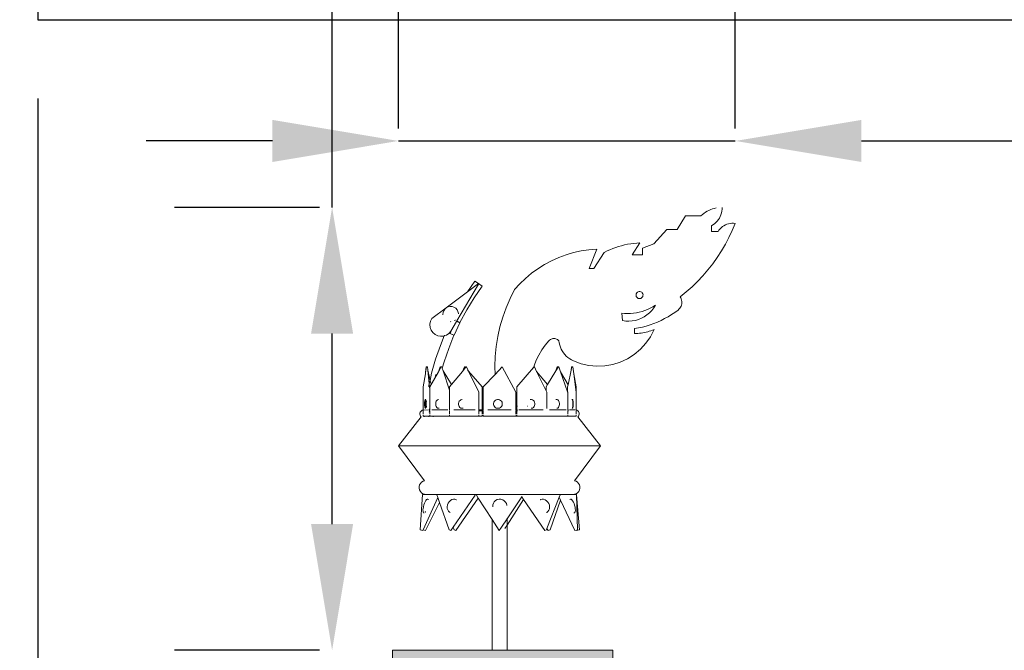
# Model space of a CAD drawing. Units: millimetres. Extents: x 7894 to 8038, y 6851 to 6951.
# Tile 44 of 49: x 7942.814 to 7950.619, y 6931.885 to 6936.88. Entities that reach past the tile are written whole.
import ezdxf

# ---------------------------------------------------------------- set-up
doc = ezdxf.new("R2010")
doc.units = ezdxf.units.MM
for name, color, linetype, lineweight in [('A-ANNO-DIMS', 2, 'Continuous', 18), ('A-FURN-ACCS', 8, 'Continuous', 13), ('A-FURN-SHLF', 7, 'Continuous', 30)]:
    doc.layers.add(name, color=color, linetype=linetype, lineweight=lineweight)
doc.layers.add('A-FURN-ACCS-PATT', color=116, linetype='Continuous', lineweight=9, true_color=0x136734)
doc.styles.get("Standard").update_dxf_attribs({"font": 'arial.ttf'})
doc.dimstyles.new('ISO-25', dxfattribs={"dimtxt": 1, "dimasz": 1, "dimexe": 1.25, "dimexo": 0.625, "dimtad": 1, "dimdec": 0, "dimlunit": 4, "dimtxsty": 'Standard', "dimcen": 2.5, "dimclrt": 1, "dimadec": 0, "dimazin": 0, "dimtfac": 1, "dimtdec": 0, "dimtmove": 0, "dimatfit": 3, "dimfxl": 1, "dimarcsym": 0})

# ---------------------------------------------------------------- blocks, each defined once
blk = doc.blocks.new('FLOATING-SHELF-ELEV')
for p, q in [((0, 0.5), (0, 0)), ((0, 0), (17.3035, 0))]:
    blk.add_line(p, q)
blk = doc.blocks.new('DISPLAY-LEAF-FINIAL')
for p, q in [((2.2094, 3.3343), (2.2756, 3.4413)), ((2.2756, 3.4413), (2.398, 3.4413)), ((2.398, 3.4413), (2.4094, 3.4516)), ((2.4094, 3.4516), (2.4214, 3.4612)), ((2.4214, 3.4612), (2.4341, 3.4699)), ((2.4341, 3.4699), (2.4472, 3.4778)), ((2.4472, 3.4778), (2.4609, 3.4849)), ((2.4609, 3.4849), (2.475, 3.4911)), ((2.475, 3.4911), (2.4894, 3.4964)), ((2.4894, 3.4964), (2.5041, 3.5007)), ((2.5041, 3.5007), (2.5191, 3.5041)), ((2.5507, 3.4368), (2.5438, 3.4237)), ((2.5562, 3.4504), (2.5507, 3.4368)), ((2.5605, 3.4646), (2.5562, 3.4504)), ((2.5634, 3.479), (2.5605, 3.4646)), ((2.5649, 3.4937), (2.5634, 3.479)), ((2.565, 3.5085), (2.5649, 3.4937)), ((2.4932, 3.3709), (2.4804, 3.3635)), ((2.4804, 3.3635), (2.4804, 3.3164)), ((2.5053, 3.3794), (2.4932, 3.3709)), ((2.5164, 3.3891), (2.5053, 3.3794)), ((2.5266, 3.3997), (2.5164, 3.3891)), ((2.5358, 3.4113), (2.5266, 3.3997)), ((2.5438, 3.4237), (2.5358, 3.4113)), ((2.5687, 3.3558), (2.5799, 3.3633)), ((2.5799, 3.3633), (2.5917, 3.3696)), ((2.5917, 3.3696), (2.604, 3.3748)), ((2.604, 3.3748), (2.6168, 3.3788)), ((2.6168, 3.3788), (2.63, 3.3815)), ((2.63, 3.3815), (2.6433, 3.3829)), ((2.6433, 3.3829), (2.6567, 3.3831)), ((2.6701, 3.3819), (2.6462, 3.3254)), ((2.6567, 3.3831), (2.6701, 3.3819)), ((2.0233, 3.2209), (2.1272, 3.3343)), ((2.1272, 3.3343), (2.2094, 3.3343)), ((2.4804, 3.3164), (2.5329, 3.3164)), ((2.5329, 3.3164), (2.5404, 3.3275)), ((2.5404, 3.3275), (2.5489, 3.3378)), ((2.5489, 3.3378), (2.5584, 3.3473)), ((2.5584, 3.3473), (2.5687, 3.3558)), ((2.6462, 3.3254), (2.6199, 3.27)), ((1.7453, 3.1982), (1.7688, 3.2049)), ((1.7688, 3.2049), (1.7926, 3.2108)), ((1.7926, 3.2108), (1.8166, 3.2158)), ((1.8166, 3.2158), (1.8408, 3.2199)), ((1.8408, 3.2199), (1.8651, 3.2232)), ((1.9139, 3.2271), (1.8536, 3.1329)), ((1.8651, 3.2232), (1.8895, 3.2256)), ((1.8895, 3.2256), (1.9139, 3.2271)), ((1.934, 3.1854), (2.0233, 3.2209)), ((2.5912, 3.2159), (2.56, 3.1631)), ((2.6199, 3.27), (2.5912, 3.2159)), ((1.2698, 3.1109), (1.3282, 3.1326)), ((1.3282, 3.1326), (1.3879, 3.1503)), ((1.3879, 3.1503), (1.4487, 3.1639)), ((1.4487, 3.1639), (1.5102, 3.1734)), ((1.5102, 3.1734), (1.5723, 3.1786)), ((1.5723, 3.1786), (1.5113, 3.0242)), ((1.5498, 3.0242), (1.6318, 3.1522)), ((1.6318, 3.1522), (1.6538, 3.163)), ((1.6538, 3.163), (1.6762, 3.173)), ((1.6762, 3.173), (1.6989, 3.1822)), ((1.6989, 3.1822), (1.7219, 3.1906)), ((1.7219, 3.1906), (1.7453, 3.1982)), ((1.8536, 3.1329), (1.934, 3.1329)), ((1.934, 3.1329), (1.934, 3.1854)), ((2.56, 3.1631), (2.5265, 3.1117)), ((1.1053, 3.0227), (1.1581, 3.0558)), ((1.1581, 3.0558), (1.213, 3.0852)), ((1.213, 3.0852), (1.2698, 3.1109)), ((2.4908, 3.0619), (2.4529, 3.0137)), ((2.5265, 3.1117), (2.4908, 3.0619)), ((1.0071, 2.9462), (1.0549, 2.9861)), ((1.0549, 2.9861), (1.1053, 3.0227)), ((1.5113, 3.0242), (1.5498, 3.0242)), ((2.4129, 2.9672), (2.3708, 2.9226)), ((2.4529, 3.0137), (2.4129, 2.9672)), ((0.634, 2.9001), (0.4633, 2.6089)), ((0.6052, 2.9243), (0.5471, 2.8395)), ((0.634, 2.9046), (0.5471, 2.8395)), ((0.634, 2.9046), (0.6052, 2.9243)), ((0.634, 2.9001), (0.634, 2.9046)), ((0.6629, 2.8848), (0.634, 2.9046)), ((0.9202, 2.857), (0.9622, 2.9031)), ((0.9622, 2.9031), (1.0071, 2.9462)), ((2.3708, 2.9226), (2.3268, 2.8799)), ((0.5471, 2.8395), (0.379, 2.7129)), ((0.5989, 2.7915), (0.6629, 2.8848)), ((0.9202, 2.857), (0.8844, 2.7861)), ((1.8829, 2.8172), (1.8849, 2.8243)), ((1.8829, 2.8099), (1.8829, 2.8172)), ((1.8849, 2.8243), (1.8885, 2.8306)), ((1.8885, 2.8306), (1.8937, 2.8357)), ((1.8937, 2.8357), (1.9001, 2.8393)), ((1.9001, 2.8393), (1.9071, 2.8412)), ((1.9071, 2.8412), (1.9144, 2.8411)), ((1.9144, 2.8411), (1.9215, 2.8392)), ((1.9215, 2.8392), (1.9278, 2.8355)), ((1.9278, 2.8355), (1.9329, 2.8303)), ((1.9329, 2.8303), (1.9365, 2.824)), ((1.9365, 2.824), (1.9384, 2.8169)), ((1.9384, 2.8169), (1.9383, 2.8096)), ((2.281, 2.8392), (2.2333, 2.8006)), ((2.3268, 2.8799), (2.281, 2.8392)), ((0.5406, 2.6956), (0.5989, 2.7915)), ((0.8844, 2.7861), (0.853, 2.7132)), ((1.8847, 2.8029), (1.8829, 2.8099)), ((1.8884, 2.7965), (1.8847, 2.8029)), ((1.8935, 2.7913), (1.8884, 2.7965)), ((1.8998, 2.7877), (1.8935, 2.7913)), ((1.9068, 2.7857), (1.8998, 2.7877)), ((1.9141, 2.7857), (1.9068, 2.7857)), ((1.9212, 2.7875), (1.9141, 2.7857)), ((1.9275, 2.7912), (1.9212, 2.7875)), ((1.9327, 2.7963), (1.9275, 2.7912)), ((1.9364, 2.8026), (1.9327, 2.7963)), ((1.9383, 2.8096), (1.9364, 2.8026)), ((2.0364, 2.7343), (2.0167, 2.7218)), ((2.0364, 2.7343), (2.023, 2.7124)), ((2.2333, 2.8006), (2.2382, 2.7921)), ((2.2382, 2.7921), (2.242, 2.7831)), ((2.243, 2.7351), (2.2397, 2.7259)), ((2.242, 2.7831), (2.2446, 2.7737)), ((2.2452, 2.7446), (2.243, 2.7351)), ((2.2446, 2.7737), (2.246, 2.764)), ((2.2462, 2.7543), (2.2452, 2.7446)), ((2.246, 2.764), (2.2462, 2.7543)), ((0.379, 2.7129), (0.2638, 2.6275)), ((0.3526, 2.6596), (0.3535, 2.675)), ((0.3527, 2.6591), (0.3526, 2.6596)), ((0.3526, 2.6569), (0.3527, 2.6591)), ((0.3535, 2.675), (0.3584, 2.6897)), ((0.3584, 2.6897), (0.3671, 2.7026)), ((0.3671, 2.7026), (0.379, 2.7129)), ((0.379, 2.7129), (0.3932, 2.7199)), ((0.3932, 2.7199), (0.4088, 2.7231)), ((0.4088, 2.7231), (0.4248, 2.7223)), ((0.4248, 2.7223), (0.44, 2.7176)), ((0.44, 2.7176), (0.4533, 2.7092)), ((0.4533, 2.7092), (0.464, 2.6977)), ((0.464, 2.6977), (0.4713, 2.6839)), ((0.4713, 2.6839), (0.4746, 2.6689)), ((0.4745, 2.6667), (0.4746, 2.6689)), ((0.4745, 2.6667), (0.4746, 2.6661)), ((0.5406, 2.6956), (0.4875, 2.5967)), ((0.853, 2.7132), (0.8261, 2.6384)), ((1.793, 2.6675), (1.7698, 2.6695)), ((1.7698, 2.6695), (1.7755, 2.6114)), ((1.8164, 2.6669), (1.793, 2.6675)), ((1.8397, 2.6677), (1.8164, 2.6669)), ((1.863, 2.6698), (1.8397, 2.6677)), ((1.886, 2.6733), (1.863, 2.6698)), ((1.9089, 2.6781), (1.886, 2.6733)), ((1.9314, 2.6843), (1.9089, 2.6781)), ((1.9535, 2.6918), (1.9314, 2.6843)), ((1.97, 2.6568), (1.9487, 2.6423)), ((1.9751, 2.7005), (1.9535, 2.6918)), ((1.9896, 2.6734), (1.97, 2.6568)), ((1.9962, 2.7106), (1.9751, 2.7005)), ((2.0073, 2.692), (1.9896, 2.6734)), ((2.0167, 2.7218), (1.9962, 2.7106)), ((2.023, 2.7124), (2.0073, 2.692)), ((2.1643, 2.6592), (2.1374, 2.6427)), ((2.1904, 2.6768), (2.1643, 2.6592)), ((2.2158, 2.6954), (2.1904, 2.6768)), ((2.2231, 2.7019), (2.2158, 2.6954)), ((2.2296, 2.7092), (2.2231, 2.7019)), ((2.2352, 2.7172), (2.2296, 2.7092)), ((2.2397, 2.7259), (2.2352, 2.7172)), ((0.2535, 2.6069), (0.2491, 2.5845)), ((0.2491, 2.58), (0.2491, 2.5845)), ((0.2491, 2.58), (0.2508, 2.5572)), ((0.2638, 2.6275), (0.2535, 2.6069)), ((0.4145, 2.6055), (0.4132, 2.6029)), ((0.4608, 2.6047), (0.4152, 2.527)), ((0.4402, 2.4957), (0.4858, 2.593)), ((0.4431, 2.613), (0.4459, 2.6117)), ((0.4509, 2.6151), (0.4489, 2.6161)), ((0.4633, 2.6089), (0.4608, 2.6047)), ((0.4858, 2.593), (0.4608, 2.6047)), ((0.4633, 2.6089), (0.4875, 2.5967)), ((0.8261, 2.6384), (0.804, 2.5621)), ((1.801, 2.6079), (1.7755, 2.6114)), ((1.8266, 2.607), (1.801, 2.6079)), ((1.8523, 2.6088), (1.8266, 2.607)), ((1.8776, 2.6133), (1.8523, 2.6088)), ((1.9023, 2.6204), (1.8776, 2.6133)), ((1.9261, 2.6301), (1.9023, 2.6204)), ((1.9487, 2.6423), (1.9261, 2.6301)), ((1.9942, 2.5779), (1.9641, 2.5686)), ((2.0239, 2.5884), (1.9942, 2.5779)), ((2.0531, 2.6002), (2.0239, 2.5884)), ((2.0818, 2.6131), (2.0531, 2.6002)), ((2.1099, 2.6273), (2.0818, 2.6131)), ((2.1374, 2.6427), (2.1099, 2.6273)), ((0.2508, 2.5572), (0.2586, 2.5356)), ((0.2586, 2.5356), (0.2719, 2.5167)), ((0.2719, 2.5167), (0.2898, 2.5018)), ((0.2898, 2.5018), (0.3111, 2.4919)), ((0.3802, 2.4968), (0.3998, 2.5097)), ((0.3983, 2.5132), (0.4016, 2.5117)), ((0.3998, 2.5097), (0.4016, 2.5117)), ((0.4029, 2.5132), (0.4004, 2.5144)), ((0.4016, 2.5117), (0.4029, 2.5132)), ((0.4016, 2.5117), (0.4399, 2.495)), ((0.4029, 2.5132), (0.4152, 2.527)), ((0.4029, 2.5132), (0.4402, 2.4957)), ((0.4085, 2.5106), (0.4078, 2.509)), ((0.4202, 2.5355), (0.4085, 2.5106)), ((0.804, 2.5621), (0.7866, 2.4847)), ((1.9029, 2.5538), (1.8718, 2.5484)), ((1.8718, 2.5484), (1.8718, 2.5082)), ((1.8718, 2.5082), (1.885, 2.5088)), ((1.885, 2.5088), (1.8981, 2.5098)), ((1.8981, 2.5098), (1.9112, 2.5112)), ((1.9336, 2.5606), (1.9029, 2.5538)), ((1.9112, 2.5112), (1.9243, 2.513)), ((1.9243, 2.513), (1.9373, 2.5152)), ((1.9641, 2.5686), (1.9336, 2.5606)), ((1.9373, 2.5152), (1.9502, 2.5177)), ((1.9502, 2.5177), (1.9631, 2.5206)), ((1.9631, 2.5206), (1.9758, 2.5239)), ((1.9758, 2.5239), (1.9885, 2.5276)), ((1.9885, 2.5276), (2.001, 2.5317)), ((2.0257, 2.5409), (1.9968, 2.4843)), ((2.001, 2.5317), (2.0134, 2.5361)), ((2.0134, 2.5361), (2.0257, 2.5409)), ((0.3111, 2.4919), (0.3343, 2.4876)), ((0.3628, 2.4909), (0.3323, 2.4155)), ((0.3343, 2.4876), (0.3579, 2.4893)), ((0.3579, 2.4893), (0.3628, 2.4909)), ((0.3628, 2.4909), (0.3802, 2.4968)), ((0.3649, 2.4962), (0.3628, 2.4909)), ((0.3978, 2.391), (0.4399, 2.495)), ((0.7866, 2.4847), (0.774, 2.4062)), ((1.1928, 2.4521), (1.1631, 2.4165)), ((1.1981, 2.4572), (1.1928, 2.4521)), ((1.2041, 2.4615), (1.1981, 2.4572)), ((1.2106, 2.465), (1.2041, 2.4615)), ((1.2175, 2.4675), (1.2106, 2.465)), ((1.2247, 2.469), (1.2175, 2.4675)), ((1.2321, 2.4695), (1.2247, 2.469)), ((1.2395, 2.469), (1.2321, 2.4695)), ((1.2467, 2.4675), (1.2395, 2.469)), ((1.2536, 2.465), (1.2467, 2.4675)), ((1.2601, 2.4615), (1.2536, 2.465)), ((1.2661, 2.4572), (1.2601, 2.4615)), ((1.2714, 2.4521), (1.2661, 2.4572)), ((1.274, 2.435), (1.2714, 2.4521)), ((1.278, 2.4183), (1.274, 2.435)), ((1.9607, 2.4321), (1.918, 2.3851)), ((1.9968, 2.4843), (1.9607, 2.4321)), ((0.3323, 2.4155), (0.2946, 2.3057)), ((0.3614, 2.2848), (0.3978, 2.391)), ((0.774, 2.4062), (0.7662, 2.3272)), ((1.1364, 2.3787), (1.1127, 2.339)), ((1.1631, 2.4165), (1.1364, 2.3787)), ((1.2834, 2.4019), (1.278, 2.4183)), ((1.2903, 2.3861), (1.2834, 2.4019)), ((1.2985, 2.371), (1.2903, 2.3861)), ((1.308, 2.3566), (1.2985, 2.371)), ((1.3187, 2.3431), (1.308, 2.3566)), ((1.3305, 2.3306), (1.3187, 2.3431)), ((1.8695, 2.3441), (1.8161, 2.3099)), ((1.918, 2.3851), (1.8695, 2.3441)), ((0.2946, 2.3057), (0.263, 2.1941)), ((0.3472, 2.2349), (0.3614, 2.2848)), ((0.7662, 2.3272), (0.7634, 2.2478)), ((1.0923, 2.2975), (1.0752, 2.2545)), ((1.1127, 2.339), (1.0923, 2.2975)), ((1.3434, 2.3192), (1.3305, 2.3306)), ((1.3572, 2.3089), (1.3434, 2.3192)), ((1.3719, 2.2999), (1.3572, 2.3089)), ((1.3873, 2.2921), (1.3719, 2.2999)), ((1.4469, 2.2701), (1.3873, 2.2921)), ((1.5088, 2.256), (1.4469, 2.2701)), ((1.698, 2.2639), (1.6355, 2.2529)), ((1.7585, 2.283), (1.698, 2.2639)), ((1.8161, 2.3099), (1.7585, 2.283)), ((0.2133, 2.1901), (0.1946, 2.0859)), ((0.2133, 2.1901), (0.2147, 2.201)), ((0.2147, 2.201), (0.2202, 2.2445)), ((0.223, 2.2445), (0.2147, 2.201)), ((0.223, 2.2445), (0.2202, 2.2445)), ((0.223, 2.2445), (0.2299, 2.2445)), ((0.2325, 2.2195), (0.2299, 2.2445)), ((0.2325, 2.2195), (0.2504, 2.1381)), ((0.2439, 2.1095), (0.2325, 2.2195)), ((0.3171, 2.2068), (0.2485, 2.0859)), ((0.263, 2.1941), (0.2504, 2.1381)), ((0.3171, 2.2068), (0.3302, 2.2445)), ((0.3385, 2.2445), (0.3171, 2.2068)), ((0.3318, 2.2445), (0.3302, 2.2445)), ((0.3441, 2.2445), (0.3385, 2.2445)), ((0.3472, 2.2349), (0.3441, 2.2445)), ((0.3543, 2.2133), (0.3472, 2.2349)), ((0.3543, 2.2133), (0.4197, 2.1042)), ((0.4044, 2.0607), (0.3543, 2.2133)), ((0.5072, 2.2093), (0.4197, 2.1042)), ((0.5072, 2.2093), (0.5246, 2.2445)), ((0.5322, 2.2392), (0.5072, 2.2093)), ((0.5277, 2.2445), (0.5246, 2.2445)), ((0.5277, 2.2445), (0.5322, 2.2392)), ((0.5366, 2.2445), (0.5322, 2.2392)), ((0.5399, 2.2445), (0.5366, 2.2445)), ((0.5559, 2.2114), (0.5399, 2.2445)), ((0.5482, 2.2204), (0.5559, 2.2114)), ((0.5559, 2.2114), (0.6628, 2.0859)), ((0.636, 2.0453), (0.5559, 2.2114)), ((0.7651, 2.1857), (0.6705, 2.0859)), ((0.7634, 2.2478), (0.7651, 2.1857)), ((0.8207, 2.2445), (0.7651, 2.1857)), ((0.93, 2.0453), (0.8207, 2.2445)), ((1.0703, 2.2388), (0.9394, 2.0859)), ((1.0703, 2.2388), (1.069, 2.2345)), ((1.0707, 2.2401), (1.0703, 2.2388)), ((1.0703, 2.2388), (1.0715, 2.2374)), ((1.0752, 2.2545), (1.0707, 2.2401)), ((1.0745, 2.2445), (1.0707, 2.2401)), ((1.0745, 2.2445), (1.0775, 2.2445)), ((1.0949, 2.2093), (1.0775, 2.2445)), ((1.0949, 2.2093), (1.1824, 2.1042)), ((1.0949, 2.2093), (1.1714, 2.0542)), ((1.2478, 2.2133), (1.1824, 2.1042)), ((1.2478, 2.2133), (1.2581, 2.2445)), ((1.2651, 2.2421), (1.2478, 2.2133)), ((1.2581, 2.2445), (1.2637, 2.2445)), ((1.2637, 2.2445), (1.2651, 2.2421)), ((1.2666, 2.2445), (1.2651, 2.2421)), ((1.2666, 2.2445), (1.272, 2.2445)), ((1.2851, 2.2068), (1.272, 2.2445)), ((1.2851, 2.2068), (1.3441, 2.1028)), ((1.2851, 2.2068), (1.3403, 2.0478)), ((1.3697, 2.2195), (1.3441, 2.1028)), ((1.3697, 2.2195), (1.3722, 2.2445)), ((1.3751, 2.2445), (1.3697, 2.2195)), ((1.3722, 2.2445), (1.3751, 2.2445)), ((1.3751, 2.2445), (1.3819, 2.2445)), ((1.3819, 2.2445), (1.3889, 2.1901)), ((1.3889, 2.1901), (1.4075, 2.0859)), ((1.4073, 2.0453), (1.3889, 2.1901)), ((1.572, 2.2503), (1.5088, 2.256)), ((1.6355, 2.2529), (1.572, 2.2503)), ((0.2439, 2.1095), (0.2392, 2.0887)), ((0.2504, 2.1381), (0.2439, 2.1095)), ((0.2485, 2.0654), (0.2439, 2.1095)), ((0.2504, 2.1381), (0.2555, 2.1145)), ((0.2969, 2.1855), (0.2916, 2.1618)), ((0.1946, 2.0859), (0.1952, 2.0478)), ((0.1949, 2.0453), (0.1946, 1.903)), ((0.1949, 2.0453), (0.1952, 2.0478)), ((0.2485, 2.0859), (0.2485, 2.0654)), ((0.2485, 2.0654), (0.2485, 1.9035)), ((0.4197, 2.1042), (0.4044, 2.0859)), ((0.4044, 2.0859), (0.4044, 2.0607)), ((0.4044, 2.0607), (0.4044, 1.9015)), ((0.636, 2.0453), (0.6371, 1.9035)), ((0.6628, 2.0859), (0.6628, 1.9035)), ((0.6705, 2.0859), (0.6705, 1.9035)), ((0.93, 2.0453), (0.9309, 1.9342)), ((0.9394, 2.0859), (0.9394, 1.9343)), ((1.1824, 2.1042), (1.1714, 2.0859)), ((1.1714, 2.0859), (1.1714, 2.0542)), ((1.1758, 2.0453), (1.1714, 2.0542)), ((1.1758, 2.0453), (1.1768, 1.9142)), ((1.3441, 2.1028), (1.3403, 2.0859)), ((1.3403, 2.0859), (1.3403, 2.0478)), ((1.3412, 2.0453), (1.3403, 2.0478)), ((1.3412, 2.0453), (1.342, 1.9035)), ((1.4075, 2.0859), (1.4073, 2.0453)), ((1.4073, 2.0453), (1.4075, 1.903)), ((0.2069, 1.956), (0.2074, 1.9648)), ((0.2069, 1.9469), (0.2069, 1.956)), ((0.2074, 1.9648), (0.2082, 1.9727)), ((0.2082, 1.9727), (0.2095, 1.9791)), ((0.2095, 1.9791), (0.211, 1.9837)), ((0.2103, 1.9469), (0.2104, 1.956)), ((0.2104, 1.956), (0.2108, 1.9648)), ((0.2108, 1.9648), (0.2117, 1.9727)), ((0.211, 1.9837), (0.2126, 1.986)), ((0.2117, 1.9727), (0.2129, 1.9791)), ((0.2161, 1.986), (0.2126, 1.986)), ((0.2129, 1.9791), (0.2144, 1.9837)), ((0.2144, 1.9837), (0.2161, 1.986)), ((0.2168, 1.9646), (0.2163, 1.9558)), ((0.2163, 1.9558), (0.2163, 1.9467)), ((0.2179, 1.9725), (0.2168, 1.9646)), ((0.218, 1.9665), (0.2168, 1.9646)), ((0.2194, 1.979), (0.2179, 1.9725)), ((0.2179, 1.9725), (0.218, 1.9665)), ((0.2202, 1.9812), (0.2194, 1.979)), ((0.2204, 1.9806), (0.2194, 1.979)), ((0.2202, 1.9646), (0.2197, 1.9558)), ((0.2197, 1.9558), (0.2197, 1.9467)), ((0.2213, 1.9725), (0.2202, 1.9646)), ((0.2218, 1.9746), (0.2213, 1.9725)), ((0.2955, 1.956), (0.2969, 1.9648)), ((0.2955, 1.9469), (0.2955, 1.956)), ((0.2969, 1.9648), (0.2997, 1.9727)), ((0.2997, 1.9727), (0.3035, 1.9791)), ((0.3035, 1.9791), (0.3083, 1.9837)), ((0.3083, 1.9837), (0.3136, 1.986)), ((0.3164, 1.986), (0.3136, 1.986)), ((0.4759, 1.956), (0.478, 1.9648)), ((0.4759, 1.9469), (0.4759, 1.956)), ((0.478, 1.9648), (0.482, 1.9727)), ((0.482, 1.9727), (0.4877, 1.9791)), ((0.4877, 1.9791), (0.4947, 1.9837)), ((0.4947, 1.9837), (0.5025, 1.986)), ((0.5041, 1.986), (0.5025, 1.986)), ((0.7536, 1.9469), (0.7537, 1.956)), ((0.7537, 1.956), (0.756, 1.9648)), ((0.756, 1.9648), (0.7606, 1.9727)), ((0.7606, 1.9727), (0.7671, 1.9791)), ((0.7671, 1.9791), (0.775, 1.9837)), ((0.775, 1.9837), (0.7838, 1.986)), ((0.7838, 1.986), (0.793, 1.986)), ((0.793, 1.986), (0.8018, 1.9836)), ((0.8018, 1.9836), (0.8096, 1.979)), ((0.8096, 1.979), (0.8161, 1.9725)), ((0.8161, 1.9725), (0.8206, 1.9646)), ((0.8206, 1.9646), (0.823, 1.9558)), ((0.823, 1.9558), (0.8229, 1.9467)), ((1.0443, 1.986), (1.0459, 1.986)), ((1.0459, 1.986), (1.0541, 1.986)), ((1.0541, 1.986), (1.062, 1.9836)), ((1.062, 1.9836), (1.0691, 1.979)), ((1.0691, 1.979), (1.0749, 1.9725)), ((1.0749, 1.9725), (1.079, 1.9646)), ((1.079, 1.9646), (1.0811, 1.9558)), ((1.0811, 1.9558), (1.0811, 1.9467)), ((1.2486, 1.986), (1.2513, 1.986)), ((1.2513, 1.986), (1.2571, 1.986)), ((1.2571, 1.986), (1.2627, 1.9836)), ((1.2627, 1.9836), (1.2677, 1.979)), ((1.2677, 1.979), (1.2717, 1.9725)), ((1.2717, 1.9725), (1.2746, 1.9646)), ((1.2746, 1.9646), (1.2761, 1.9558)), ((1.2761, 1.9558), (1.2761, 1.9467)), ((1.3734, 1.986), (1.3755, 1.986)), ((1.3755, 1.986), (1.3775, 1.9836)), ((1.3755, 1.986), (1.3768, 1.986)), ((1.3768, 1.986), (1.3789, 1.986)), ((1.3775, 1.9836), (1.3794, 1.979)), ((1.3789, 1.986), (1.3809, 1.9836)), ((1.3794, 1.979), (1.3809, 1.9725)), ((1.3809, 1.9836), (1.3828, 1.979)), ((1.3809, 1.9725), (1.3819, 1.9646)), ((1.3819, 1.9646), (1.3825, 1.9558)), ((1.3825, 1.9558), (1.3825, 1.9467)), ((1.3828, 1.979), (1.3843, 1.9725)), ((1.3843, 1.9725), (1.3853, 1.9646)), ((1.3853, 1.9646), (1.3859, 1.9558)), ((1.3859, 1.9558), (1.3859, 1.9467)), ((0.1696, 1.8695), (0.1697, 1.8775)), ((0.1697, 1.8775), (0.1719, 1.8852)), ((0.1719, 1.8852), (0.176, 1.892)), ((0.176, 1.892), (0.1817, 1.8976)), ((0.1817, 1.8976), (0.1887, 1.9015)), ((0.1887, 1.9015), (0.1946, 1.903)), ((0.1946, 1.8976), (0.1945, 1.8695)), ((0.1946, 1.903), (0.1964, 1.9035)), ((0.1946, 1.903), (0.1946, 1.9015)), ((0.1964, 1.9035), (0.1977, 1.9034)), ((0.1964, 1.9035), (0.1969, 1.9035)), ((0.2373, 1.9035), (0.1977, 1.9034)), ((0.2074, 1.938), (0.2069, 1.9469)), ((0.2082, 1.9301), (0.2074, 1.938)), ((0.2094, 1.9236), (0.2082, 1.9301)), ((0.2109, 1.9191), (0.2094, 1.9236)), ((0.2108, 1.938), (0.2103, 1.9469)), ((0.2116, 1.9301), (0.2108, 1.938)), ((0.2126, 1.9167), (0.2109, 1.9191)), ((0.2129, 1.9236), (0.2116, 1.9301)), ((0.2143, 1.9167), (0.2126, 1.9167)), ((0.2163, 1.9467), (0.2129, 1.9236)), ((0.2144, 1.9191), (0.2129, 1.9236)), ((0.216, 1.9167), (0.2143, 1.9167)), ((0.216, 1.9167), (0.2144, 1.9191)), ((0.2177, 1.9167), (0.216, 1.9167)), ((0.2163, 1.9467), (0.2168, 1.9379)), ((0.2168, 1.9379), (0.2179, 1.93)), ((0.2179, 1.93), (0.2194, 1.9235)), ((0.2194, 1.9235), (0.2202, 1.9215)), ((0.2197, 1.9467), (0.2202, 1.9379)), ((0.2202, 1.9379), (0.2213, 1.93)), ((0.2213, 1.93), (0.2218, 1.928)), ((0.2485, 1.9035), (0.2439, 1.9035)), ((0.2485, 1.8971), (0.2439, 1.8971)), ((0.2453, 1.8976), (0.244, 1.8856)), ((0.2485, 1.9251), (0.2458, 1.9015)), ((0.2485, 1.9035), (0.2485, 1.9015)), ((0.2485, 1.8976), (0.2485, 1.8971)), ((0.2485, 1.8971), (0.2485, 1.8695)), ((0.3913, 1.9035), (0.265, 1.9035)), ((0.2969, 1.938), (0.2955, 1.9469)), ((0.2996, 1.9301), (0.2969, 1.938)), ((0.3034, 1.9236), (0.2996, 1.9301)), ((0.3082, 1.9191), (0.3034, 1.9236)), ((0.3134, 1.9167), (0.3082, 1.9191)), ((0.3189, 1.9167), (0.3134, 1.9167)), ((0.3217, 1.9167), (0.3189, 1.9167)), ((0.4044, 1.8976), (0.4044, 1.8695)), ((0.4385, 1.9035), (0.6066, 1.9035)), ((0.478, 1.938), (0.4759, 1.9469)), ((0.4819, 1.9301), (0.478, 1.938)), ((0.4876, 1.9236), (0.4819, 1.9301)), ((0.4945, 1.9191), (0.4876, 1.9236)), ((0.5023, 1.9167), (0.4945, 1.9191)), ((0.5103, 1.9167), (0.5023, 1.9167)), ((0.512, 1.9167), (0.5103, 1.9167)), ((0.6371, 1.9035), (0.6338, 1.9035)), ((0.6371, 1.8971), (0.6338, 1.8971)), ((0.6371, 1.9035), (0.6371, 1.9015)), ((0.6628, 1.9035), (0.6371, 1.9035)), ((0.6371, 1.8976), (0.6371, 1.8971)), ((0.6371, 1.8971), (0.6374, 1.8695)), ((0.6628, 1.8971), (0.6371, 1.8971)), ((0.6628, 1.9035), (0.6705, 1.9035)), ((0.6628, 1.9035), (0.6628, 1.9015)), ((0.6628, 1.8976), (0.6628, 1.8971)), ((0.6628, 1.8971), (0.6628, 1.8695)), ((0.6705, 1.8971), (0.6628, 1.8971)), ((0.6705, 1.9035), (0.6705, 1.9015)), ((0.6705, 1.8976), (0.6705, 1.8971)), ((0.6705, 1.8971), (0.6705, 1.8695)), ((0.7081, 1.9035), (0.894, 1.9035)), ((0.756, 1.938), (0.7536, 1.9469)), ((0.7605, 1.9301), (0.756, 1.938)), ((0.7669, 1.9236), (0.7605, 1.9301)), ((0.7748, 1.9191), (0.7669, 1.9236)), ((0.7836, 1.9167), (0.7748, 1.9191)), ((0.7928, 1.9167), (0.7836, 1.9167)), ((0.8016, 1.919), (0.7928, 1.9167)), ((0.8095, 1.9235), (0.8016, 1.919)), ((0.816, 1.93), (0.8095, 1.9235)), ((0.8206, 1.9379), (0.816, 1.93)), ((0.8229, 1.9467), (0.8206, 1.9379)), ((0.9394, 1.9343), (0.9309, 1.9342)), ((0.9309, 1.9342), (0.9312, 1.9035)), ((0.9312, 1.9035), (0.9312, 1.9015)), ((0.9394, 1.9035), (0.9312, 1.9035)), ((0.9313, 1.8976), (0.9313, 1.8971)), ((0.9313, 1.8971), (0.9315, 1.8695)), ((0.9394, 1.8971), (0.9313, 1.8971)), ((0.9424, 1.9343), (0.9394, 1.9343)), ((0.9394, 1.9343), (0.9394, 1.9035)), ((0.9424, 1.9035), (0.9394, 1.9035)), ((0.9394, 1.9035), (0.9394, 1.9015)), ((0.9394, 1.8976), (0.9394, 1.8971)), ((0.9424, 1.8971), (0.9394, 1.8971)), ((0.9394, 1.8971), (0.9394, 1.8695)), ((0.9534, 1.9035), (1.1456, 1.9035)), ((1.0224, 1.935), (1.0209, 1.935)), ((1.0524, 1.9167), (1.0539, 1.9167)), ((1.0618, 1.919), (1.0539, 1.9167)), ((1.069, 1.9235), (1.0618, 1.919)), ((1.0748, 1.93), (1.069, 1.9235)), ((1.0789, 1.9379), (1.0748, 1.93)), ((1.0811, 1.9467), (1.0789, 1.9379)), ((1.3304, 1.9035), (1.1965, 1.9035)), ((1.2543, 1.9167), (1.257, 1.9167)), ((1.2626, 1.919), (1.257, 1.9167)), ((1.2676, 1.9235), (1.2626, 1.919)), ((1.2717, 1.93), (1.2676, 1.9235)), ((1.2746, 1.9379), (1.2717, 1.93)), ((1.2761, 1.9467), (1.2746, 1.9379)), ((1.3471, 1.9035), (1.342, 1.9035)), ((1.342, 1.9035), (1.342, 1.9015)), ((1.342, 1.8976), (1.342, 1.8971)), ((1.3471, 1.8971), (1.342, 1.8971)), ((1.342, 1.8971), (1.3421, 1.8695)), ((1.3561, 1.9035), (1.4004, 1.9035)), ((1.3775, 1.919), (1.3755, 1.9167)), ((1.3755, 1.9167), (1.3789, 1.9167)), ((1.3793, 1.9235), (1.3775, 1.919)), ((1.3809, 1.919), (1.3789, 1.9167)), ((1.3808, 1.93), (1.3793, 1.9235)), ((1.3819, 1.9379), (1.3808, 1.93)), ((1.3827, 1.9235), (1.3809, 1.919)), ((1.3825, 1.9467), (1.3819, 1.9379)), ((1.3842, 1.93), (1.3827, 1.9235)), ((1.3853, 1.9379), (1.3842, 1.93)), ((1.3859, 1.9467), (1.3853, 1.9379)), ((1.4075, 1.903), (1.4135, 1.9015)), ((1.4075, 1.903), (1.4075, 1.9015)), ((1.4075, 1.8976), (1.4075, 1.8695)), ((1.4135, 1.9015), (1.4205, 1.8976)), ((1.4205, 1.8976), (1.4262, 1.892)), ((1.4262, 1.892), (1.4303, 1.8852)), ((1.4303, 1.8852), (1.4325, 1.8775)), ((1.4325, 1.8775), (1.4326, 1.8695)), ((0, 1.6201), (0.181, 1.8491)), ((0.1715, 1.8618), (0.1696, 1.8695)), ((0.1754, 1.8548), (0.1715, 1.8618)), ((0.181, 1.8491), (0.1754, 1.8548)), ((0.1945, 1.8618), (0.1945, 1.8548)), ((0.1952, 1.8548), (0.1945, 1.8548)), ((0.2052, 1.8548), (0.1945, 1.8548)), ((0.2048, 1.8513), (0.2047, 1.8491)), ((0.2052, 1.8548), (0.2048, 1.8513)), ((0.2485, 1.8548), (0.2052, 1.8548)), ((0.2404, 1.8548), (0.2398, 1.8491)), ((0.2485, 1.8618), (0.2485, 1.8548)), ((0.2485, 1.8548), (0.2756, 1.8548)), ((0.275, 1.8491), (0.2756, 1.8548)), ((0.2756, 1.8548), (0.4049, 1.8548)), ((0.4044, 1.8618), (0.4049, 1.8548)), ((0.4049, 1.8548), (0.6375, 1.8548)), ((0.6374, 1.8618), (0.6375, 1.8548)), ((0.6628, 1.8548), (0.6375, 1.8548)), ((0.6628, 1.8618), (0.6628, 1.8548)), ((0.6705, 1.8618), (0.6705, 1.8548)), ((0.6705, 1.8548), (0.9316, 1.8548)), ((0.9316, 1.8618), (0.9316, 1.8548)), ((0.9394, 1.8548), (0.9316, 1.8548)), ((0.9394, 1.8618), (0.9394, 1.8548)), ((1.3422, 1.8548), (0.9394, 1.8548)), ((1.3422, 1.8618), (1.3422, 1.8548)), ((1.4075, 1.8548), (1.3422, 1.8548)), ((1.4075, 1.8618), (1.4075, 1.8548)), ((1.4267, 1.8548), (1.4212, 1.8491)), ((1.4212, 1.8491), (1.6021, 1.6201)), ((1.4306, 1.8618), (1.4267, 1.8548)), ((1.4326, 1.8695), (1.4306, 1.8618)), ((0.2072, 1.3429), (0, 1.6201)), ((1.6021, 1.6201), (0, 1.6201)), ((1.6021, 1.6201), (1.395, 1.3429)), ((0.1742, 1.3213), (0.1833, 1.3311)), ((0.1833, 1.3311), (0.1945, 1.3384)), ((0.1945, 1.3384), (0.2072, 1.3429)), ((1.395, 1.3429), (1.4076, 1.3384)), ((1.4076, 1.3384), (1.4188, 1.3311)), ((1.4188, 1.3311), (1.4279, 1.3213)), ((0.1641, 1.2831), (0.1643, 1.2966)), ((0.1672, 1.2701), (0.1641, 1.2831)), ((0.1643, 1.2966), (0.1678, 1.3095)), ((0.1733, 1.2582), (0.1672, 1.2701)), ((0.1678, 1.3095), (0.1742, 1.3213)), ((0.1821, 1.2481), (0.1733, 1.2582)), ((1.4288, 1.2582), (1.42, 1.2481)), ((1.4279, 1.3213), (1.4344, 1.3095)), ((1.435, 1.2701), (1.4288, 1.2582)), ((1.4344, 1.3095), (1.4378, 1.2966)), ((1.438, 1.2831), (1.435, 1.2701)), ((1.4378, 1.2966), (1.438, 1.2831)), ((0.1714, 0.9553), (0.1907, 1.234)), ((0.1931, 1.2404), (0.1821, 1.2481)), ((0.2189, 1.234), (0.1907, 1.234)), ((0.2056, 1.2356), (0.1931, 1.2404)), ((0.1964, 0.9543), (0.3109, 1.2098)), ((0.2189, 1.234), (0.2056, 1.2356)), ((0.2065, 1.165), (0.2118, 1.177)), ((0.2118, 1.177), (0.2173, 1.1867)), ((0.2147, 0.949), (0.3244, 1.1717)), ((0.2173, 1.1867), (0.2227, 1.1934)), ((0.2189, 1.234), (0.2969, 1.234)), ((0.2227, 1.1934), (0.2276, 1.1967)), ((0.2276, 1.1967), (0.2317, 1.1963)), ((0.2325, 1.1953), (0.2317, 1.1963)), ((0.2325, 1.1953), (0.2366, 1.1949)), ((0.2969, 1.234), (0.3023, 1.234)), ((0.3029, 1.2321), (0.2969, 1.234)), ((0.3029, 1.2321), (0.3023, 1.234)), ((0.3023, 1.234), (0.5943, 1.234)), ((0.3109, 1.2098), (0.3029, 1.2321)), ((0.3244, 1.1717), (0.3109, 1.2098)), ((0.4015, 0.9553), (0.3244, 1.1717)), ((0.3948, 1.165), (0.4028, 1.177)), ((0.4028, 1.177), (0.4128, 1.1867)), ((0.4128, 1.1867), (0.4241, 1.1934)), ((0.4241, 1.1934), (0.436, 1.1967)), ((0.434, 0.9751), (0.6087, 1.2276)), ((0.436, 1.1967), (0.4475, 1.1963)), ((0.4475, 1.1963), (0.4584, 1.1919)), ((0.455, 0.949), (0.6322, 1.205)), ((0.4584, 1.1919), (0.4611, 1.1909)), ((0.5943, 1.234), (0.6175, 1.234)), ((0.6087, 1.2276), (0.5943, 1.234)), ((0.6175, 1.2276), (0.6175, 1.234)), ((0.9517, 1.234), (0.6175, 1.234)), ((0.6322, 1.205), (0.6175, 1.2276)), ((0.7416, 1.0372), (0.6322, 1.205)), ((0.752, 1.165), (0.7597, 1.177)), ((0.7597, 1.177), (0.7703, 1.1867)), ((0.7703, 1.1867), (0.7831, 1.1934)), ((0.7831, 1.1934), (0.7973, 1.1967)), ((0.7973, 1.1967), (0.8119, 1.1963)), ((0.8119, 1.1963), (0.8259, 1.1923)), ((0.8259, 1.1923), (0.8383, 1.1849)), ((0.8383, 1.1849), (0.8484, 1.1746)), ((0.8484, 1.1746), (0.8553, 1.1622)), ((0.8605, 1.0411), (0.9765, 1.2154)), ((0.8605, 0.9923), (0.9902, 1.1955)), ((0.9809, 1.2337), (0.9517, 1.234)), ((0.9765, 1.2154), (0.9744, 1.2185)), ((0.9902, 1.1955), (0.9765, 1.2154)), ((0.9809, 1.2337), (0.9815, 1.234)), ((0.9815, 1.234), (0.983, 1.234)), ((1.2836, 1.234), (0.983, 1.234)), ((1.16, 0.949), (0.9902, 1.1955)), ((1.1241, 1.1921), (1.1257, 1.1925)), ((1.1257, 1.1925), (1.127, 1.1934)), ((1.127, 1.1934), (1.1382, 1.1967)), ((1.1382, 1.1967), (1.1502, 1.1963)), ((1.1502, 1.1963), (1.1624, 1.1923)), ((1.1624, 1.1923), (1.1737, 1.1849)), ((1.1737, 1.1849), (1.1835, 1.1746)), ((1.1768, 0.964), (1.2748, 1.2121)), ((1.1835, 1.1746), (1.1911, 1.1622)), ((1.2015, 0.9553), (1.285, 1.1903)), ((1.2748, 1.2121), (1.2826, 1.2319)), ((1.285, 1.1903), (1.2748, 1.2121)), ((1.2826, 1.2319), (1.2898, 1.234)), ((1.2826, 1.2319), (1.2836, 1.234)), ((1.2836, 1.234), (1.2898, 1.234)), ((1.398, 0.949), (1.285, 1.1903)), ((1.2898, 1.234), (1.3832, 1.234)), ((1.359, 1.1953), (1.3638, 1.1967)), ((1.359, 1.1953), (1.3619, 1.1951)), ((1.3638, 1.1967), (1.3687, 1.1963)), ((1.3687, 1.1963), (1.3744, 1.1923)), ((1.3744, 1.1923), (1.3804, 1.1849)), ((1.3804, 1.1849), (1.3863, 1.1746)), ((1.3965, 1.2356), (1.3832, 1.234)), ((1.41, 1.2337), (1.3832, 1.234)), ((1.3863, 1.1746), (1.3917, 1.1622)), ((1.4091, 1.2404), (1.3965, 1.2356)), ((1.42, 1.2481), (1.4091, 1.2404)), ((1.4111, 1.234), (1.41, 1.2337)), ((1.4113, 1.2316), (1.4111, 1.234)), ((1.4348, 0.9553), (1.4113, 1.2316)), ((1.4203, 0.9553), (1.4113, 1.2316)), ((0.1943, 1.1113), (0.1955, 1.1237)), ((0.1946, 1.101), (0.1943, 1.1113)), ((0.1963, 1.0936), (0.1946, 1.101)), ((0.1955, 1.1237), (0.1981, 1.1374)), ((0.1993, 1.0896), (0.1963, 1.0936)), ((0.1981, 1.1374), (0.2018, 1.1515)), ((0.2018, 1.1515), (0.2065, 1.165)), ((0.2112, 1.0961), (0.2129, 1.0925)), ((0.2141, 1.1), (0.2145, 1.0978)), ((0.3867, 1.1374), (0.3893, 1.1515)), ((0.3871, 1.1237), (0.3867, 1.1374)), ((0.3906, 1.1113), (0.3871, 1.1237)), ((0.3893, 1.1515), (0.3948, 1.165)), ((0.3969, 1.101), (0.3906, 1.1113)), ((0.4056, 1.0936), (0.3969, 1.101)), ((0.4087, 1.0923), (0.4056, 1.0936)), ((0.7474, 1.1361), (0.7475, 1.1373)), ((0.7475, 1.1373), (0.7478, 1.1515)), ((0.7478, 1.1515), (0.752, 1.165)), ((0.8553, 1.1622), (0.8587, 1.1485)), ((0.8587, 1.1471), (0.8587, 1.1485)), ((1.1847, 1.0992), (1.1752, 1.0925)), ((1.192, 1.1089), (1.1847, 1.0992)), ((1.1911, 1.1622), (1.196, 1.1485)), ((1.1964, 1.1209), (1.192, 1.1089)), ((1.196, 1.1485), (1.1978, 1.1344)), ((1.1978, 1.1344), (1.1964, 1.1209)), ((1.3917, 1.1622), (1.3963, 1.1485)), ((1.3963, 1.1485), (1.3997, 1.1344)), ((1.4012, 1.0992), (1.3987, 1.0925)), ((1.3997, 1.1344), (1.4018, 1.1209)), ((1.4023, 1.1089), (1.4012, 1.0992)), ((1.4018, 1.1209), (1.4023, 1.1089)), ((0.2034, 1.0892), (0.1993, 1.0896)), ((0.2041, 1.0883), (0.2034, 1.0892)), ((0.2129, 1.0925), (0.2137, 1.0919)), ((0.7416, 0), (0.7416, 1.0372)), ((0.7992, 0.949), (0.7416, 1.0372)), ((0.8158, 0.974), (0.8605, 1.0411)), ((0.8605, 1.0411), (0.8605, 1.0475)), ((0.8605, 0.9923), (0.8605, 1.0411)), ((1.1736, 1.092), (1.1723, 1.0911)), ((1.1736, 1.092), (1.1752, 1.0925)), ((1.3919, 1.0894), (1.39, 1.0879)), ((1.39, 1.0879), (1.3948, 1.0892)), ((1.3987, 1.0925), (1.3948, 1.0892)), ((0.1941, 0.949), (0.1714, 0.9553)), ((0.1941, 0.949), (0.1964, 0.9543)), ((0.2147, 0.949), (0.1964, 0.9543)), ((0.4159, 0.949), (0.4015, 0.9553)), ((0.4159, 0.949), (0.434, 0.9751)), ((0.4421, 0.9553), (0.434, 0.9751)), ((0.455, 0.949), (0.4421, 0.9553)), ((0.7992, 0.949), (0.8158, 0.974)), ((0.8158, 0.974), (0.8137, 0.9772)), ((0.8165, 0.9731), (0.8158, 0.974)), ((0.8431, 0.9651), (0.8605, 0.9923)), ((0.8605, 0), (0.8605, 0.9923)), ((1.16, 0.949), (1.1734, 0.9553)), ((1.1734, 0.9553), (1.1768, 0.964)), ((1.1872, 0.949), (1.1768, 0.964)), ((1.1872, 0.949), (1.2015, 0.9553)), ((1.398, 0.949), (1.4105, 0.9525)), ((1.4105, 0.9525), (1.4203, 0.9553)), ((1.412, 0.949), (1.4105, 0.9525)), ((1.412, 0.949), (1.4348, 0.9553))]:
    blk.add_line(p, q)
blk = doc.blocks.new('*D17')
at = {"layer": 'A-ANNO-DIMS', "color": 0, "lineweight": -2, "transparency": 16777216}
for p, q in [((7945.2906, 6935.3937), (7945.2906, 6950.7481)), ((7945.1919, 6935.3937), (7944.0406, 6935.3937)), ((7945.2906, 6932.8853), (7945.2906, 6934.3937)), ((7945.1919, 6931.8853), (7944.0406, 6931.8853))]:
    blk.add_line(p, q, dxfattribs=at)
at = {"layer": 'A-ANNO-DIMS', "color": 0, "transparency": 16777216}
for points in [[(7945.124, 6934.3937), (7945.4573, 6934.3937), (7945.2906, 6935.3937)], [(7945.124, 6932.8853), (7945.4573, 6932.8853), (7945.2906, 6931.8853)]]:
    blk.add_solid(points, dxfattribs=at)
at = {"layer": 'Defpoints', "color": 0, "transparency": 16777216}
for p in [(7945.2906, 6935.3937), (7945.8169, 6935.3937), (7945.8169, 6931.8853)]:
    blk.add_point(p, dxfattribs=at)
at = {"layer": 'A-ANNO-DIMS', "color": 1, "transparency": 16777216, "insert": (7944.1482, 6943.5709), "char_height": 1, "attachment_point": 5, "rotation": 90}
blk.add_mtext('FINIAL 0\'-3 1/2" TYP.', dxfattribs=at)
blk = doc.blocks.new('*D18')
at = {"layer": 'A-ANNO-DIMS', "color": 0, "lineweight": -2, "transparency": 16777216}
for p, q in [((7945.8169, 6936.0187), (7945.8169, 6937.17)), ((7948.487, 6936.0187), (7948.487, 6937.17)), ((7944.8169, 6935.92), (7943.8169, 6935.92)), ((7945.8169, 6935.92), (7948.487, 6935.92)), ((7949.487, 6935.92), (7960.1626, 6935.92))]:
    blk.add_line(p, q, dxfattribs=at)
at = {"layer": 'A-ANNO-DIMS', "color": 0, "transparency": 16777216}
for points in [[(7944.8169, 6936.0867), (7944.8169, 6935.7534), (7945.8169, 6935.92)], [(7949.487, 6936.0867), (7949.487, 6935.7534), (7948.487, 6935.92)]]:
    blk.add_solid(points, dxfattribs=at)
at = {"layer": 'Defpoints', "color": 0, "transparency": 16777216}
for p in [(7948.487, 6935.92), (7945.8169, 6935.3937), (7948.487, 6935.3937)]:
    blk.add_point(p, dxfattribs=at)
at = {"layer": 'A-ANNO-DIMS', "color": 1, "transparency": 16777216, "insert": (7955.3248, 6937.0621), "char_height": 1, "attachment_point": 5}
blk.add_mtext('0\'-2 1/2" TYP.', dxfattribs=at)
blk = doc.blocks.new('*D23')
at = {"layer": 'A-ANNO-DIMS', "color": 0, "lineweight": -2, "transparency": 16777216}
for p, q in [((7940.0888, 6907.098), (7940.0888, 6947.7928)), ((7971.9356, 6928.989), (7971.9356, 6947.7928)), ((7941.0888, 6946.5428), (7970.9356, 6946.5428))]:
    blk.add_line(p, q, dxfattribs=at)
at = {"layer": 'A-ANNO-DIMS', "color": 0, "transparency": 16777216}
for points in [[(7941.0888, 6946.7095), (7941.0888, 6946.3762), (7940.0888, 6946.5428)], [(7970.9356, 6946.7095), (7970.9356, 6946.3762), (7971.9356, 6946.5428)]]:
    blk.add_solid(points, dxfattribs=at)
at = {"layer": 'Defpoints', "color": 0, "transparency": 16777216}
for p in [(7971.9356, 6946.5428), (7971.9356, 6928.364), (7940.0888, 6906.473)]:
    blk.add_point(p, dxfattribs=at)
at = {"layer": 'A-ANNO-DIMS', "color": 1, "transparency": 16777216, "insert": (7956.0122, 6947.6784), "char_height": 1, "attachment_point": 5}
blk.add_mtext('2\'-8"', dxfattribs=at)
blk = doc.blocks.new('*D24')
at = {"layer": 'A-ANNO-DIMS', "color": 0, "lineweight": -2, "transparency": 16777216}
for p, q in [((7953.3408, 6944.6059), (7936.9023, 6944.6059)), ((7938.1523, 6907.473), (7938.1523, 6943.6059)), ((7939.4638, 6906.473), (7936.9023, 6906.473))]:
    blk.add_line(p, q, dxfattribs=at)
at = {"layer": 'A-ANNO-DIMS', "color": 0, "transparency": 16777216}
for points in [[(7937.9856, 6943.6059), (7938.319, 6943.6059), (7938.1523, 6944.6059)], [(7937.9856, 6907.473), (7938.319, 6907.473), (7938.1523, 6906.473)]]:
    blk.add_solid(points, dxfattribs=at)
at = {"layer": 'Defpoints', "color": 0, "transparency": 16777216}
for p in [(7938.1523, 6944.6059), (7953.9658, 6944.6059), (7940.0888, 6906.473)]:
    blk.add_point(p, dxfattribs=at)
at = {"layer": 'A-ANNO-DIMS', "color": 1, "transparency": 16777216, "insert": (7937.0164, 6925.5395), "char_height": 1, "attachment_point": 5, "rotation": 90}
blk.add_mtext('3\'-2"', dxfattribs=at)
blk = doc.blocks.new('*D35')
at = {"layer": 'A-ANNO-DIMS', "color": 0, "lineweight": -2, "transparency": 16777216}
for p, q in [((7942.9569, 6936.2554), (7942.9569, 6903.2865)), ((7943.7365, 6929.5331), (7943.7365, 6903.2865)), ((7941.9569, 6904.5365), (7937.0486, 6904.5365)), ((7943.7365, 6904.5365), (7942.9569, 6904.5365)), ((7944.7365, 6904.5365), (7945.7365, 6904.5365))]:
    blk.add_line(p, q, dxfattribs=at)
at = {"layer": 'A-ANNO-DIMS', "color": 0, "transparency": 16777216}
for points in [[(7941.9569, 6904.7032), (7941.9569, 6904.3699), (7942.9569, 6904.5365)], [(7944.7365, 6904.7032), (7944.7365, 6904.3699), (7943.7365, 6904.5365)]]:
    blk.add_solid(points, dxfattribs=at)
at = {"layer": 'Defpoints', "color": 0, "transparency": 16777216}
for p in [(7942.9569, 6936.8804), (7943.7365, 6930.1581), (7942.9569, 6904.5365)]:
    blk.add_point(p, dxfattribs=at)
at = {"layer": 'A-ANNO-DIMS', "color": 1, "transparency": 16777216, "insert": (7939.0027, 6905.6721), "char_height": 1, "attachment_point": 5}
blk.add_mtext('0\'-1"', dxfattribs=at)

msp = doc.modelspace()

# ---------------------------------------------------------------- hatches: boundary and pattern name
at = {"layer": 'A-FURN-ACCS-PATT'}
h = msp.add_hatch(color=256, dxfattribs=at)
h.dxf.hatch_style = 1
h.paths.add_polyline_path([(7947.5161, 6931.8853), (7946.6774, 6931.8853), (7946.5585, 6931.8853), (7945.7683, 6931.8853), (7945.7683, 6930.1581), (7947.5161, 6930.1581)])
h.paths.add_polyline_path([(7947.4851, 6922.447), (7946.6464, 6922.447), (7946.5276, 6922.447), (7945.7373, 6922.447), (7945.7373, 6920.7198), (7947.4851, 6920.7198)])
h.paths.add_polyline_path([(7968.0212, 6935.881), (7967.1825, 6935.881), (7967.0637, 6935.881), (7966.2734, 6935.881), (7966.2734, 6934.1538), (7968.0212, 6934.1538)])
h.paths.add_polyline_path([(7960.6099, 6924.8555), (7959.7712, 6924.8555), (7959.6523, 6924.8555), (7958.862, 6924.8555), (7958.862, 6923.1283), (7960.6099, 6923.1283)])
h.paths.add_polyline_path([(7964.717, 6924.8555), (7963.8783, 6924.8555), (7963.7594, 6924.8555), (7962.9691, 6924.8555), (7962.9691, 6923.1283), (7964.717, 6923.1283)])
h.paths.add_polyline_path([(7971.0698, 6924.8555), (7970.2311, 6924.8555), (7970.1123, 6924.8555), (7969.322, 6924.8555), (7969.322, 6923.1283), (7971.0698, 6923.1283)])
h.paths.add_polyline_path([(7958.5294, 6908.7006), (7957.6907, 6908.7006), (7957.5718, 6908.7006), (7956.7815, 6908.7006), (7956.7815, 6906.9734), (7958.5294, 6906.9734)])

# ---------------------------------------------------------------- linework, layer by layer
at = {"layer": 'A-FURN-ACCS'}
for p, q in [((7945.7683, 6930.1581), (7945.7683, 6931.8853)), ((7945.7683, 6931.8853), (7946.5585, 6931.8853)), ((7946.6774, 6931.8853), (7946.5585, 6931.8853)), ((7946.6774, 6931.8853), (7947.5161, 6931.8853)), ((7947.5161, 6930.1581), (7947.5161, 6931.8853))]:
    msp.add_line(p, q, dxfattribs=at)

# ---------------------------------------------------------------- block references
msp.add_blockref('DISPLAY-LEAF-FINIAL', (7945.8169, 6931.8853), dxfattribs=at)
at = {"layer": 'A-FURN-SHLF'}
msp.add_blockref('FLOATING-SHELF-ELEV', (7942.9569, 6936.8804), dxfattribs=at)

# ---------------------------------------------------------------- dimensions: what is measured, and where the dimension line sits
at = {"layer": 'A-ANNO-DIMS'}
dim = msp.add_linear_dim(base=(7945.2906, 6935.3937), p1=(7945.8169, 6931.8853), p2=(7945.8169, 6935.3937), angle=90, text='FINIAL <> TYP.', dimstyle='ISO-25', override={"dimdec": 1, "dimlfac": 1, "dimrnd": 0, "dimzin": 1, "dimdsep": 46, "dimlunit": 4, "dimfrac": 2}, dxfattribs=at)
dim.commit()
dim.dimension.update_dxf_attribs({"geometry": '*D17', "text_midpoint": (7944.1482, 6943.5709)})
for base, p1, p2, picture, middle in [((7971.9356, 6946.5428), (7940.0888, 6906.473), (7971.9356, 6928.364), '*D23', (7956.0122, 6947.6784)), ((7942.9569, 6904.5365), (7943.7365, 6930.1581), (7942.9569, 6936.8804), '*D35', (7939.0027, 6905.6721))]:
    dim = msp.add_linear_dim(base=base, p1=p1, p2=p2, dimstyle='ISO-25', override={"dimdec": 1, "dimlfac": 1, "dimrnd": 0, "dimzin": 1, "dimdsep": 46, "dimlunit": 4, "dimfrac": 2}, dxfattribs=at)
    dim.commit()
    dim.dimension.update_dxf_attribs({"geometry": picture, "text_midpoint": middle})
dim = msp.add_linear_dim(base=(7938.1523, 6944.6059), p1=(7940.0888, 6906.473), p2=(7953.9658, 6944.6059), angle=90, dimstyle='ISO-25', override={"dimdec": 1, "dimlfac": 1, "dimrnd": 0, "dimzin": 1, "dimdsep": 46, "dimlunit": 4, "dimfrac": 2}, dxfattribs=at)
dim.commit()
dim.dimension.update_dxf_attribs({"geometry": '*D24', "text_midpoint": (7937.0164, 6925.5395)})
dim = msp.add_linear_dim(base=(7948.487, 6935.92), p1=(7945.8169, 6935.3937), p2=(7948.487, 6935.3937), text='<> TYP.', dimstyle='ISO-25', override={"dimdec": 1, "dimlfac": 1, "dimrnd": 0, "dimzin": 1, "dimdsep": 46, "dimlunit": 4, "dimfrac": 2}, dxfattribs=at)
dim.commit()
dim.dimension.update_dxf_attribs({"geometry": '*D18', "text_midpoint": (7955.3248, 6937.0621)})

doc.saveas('drawing.dxf')
